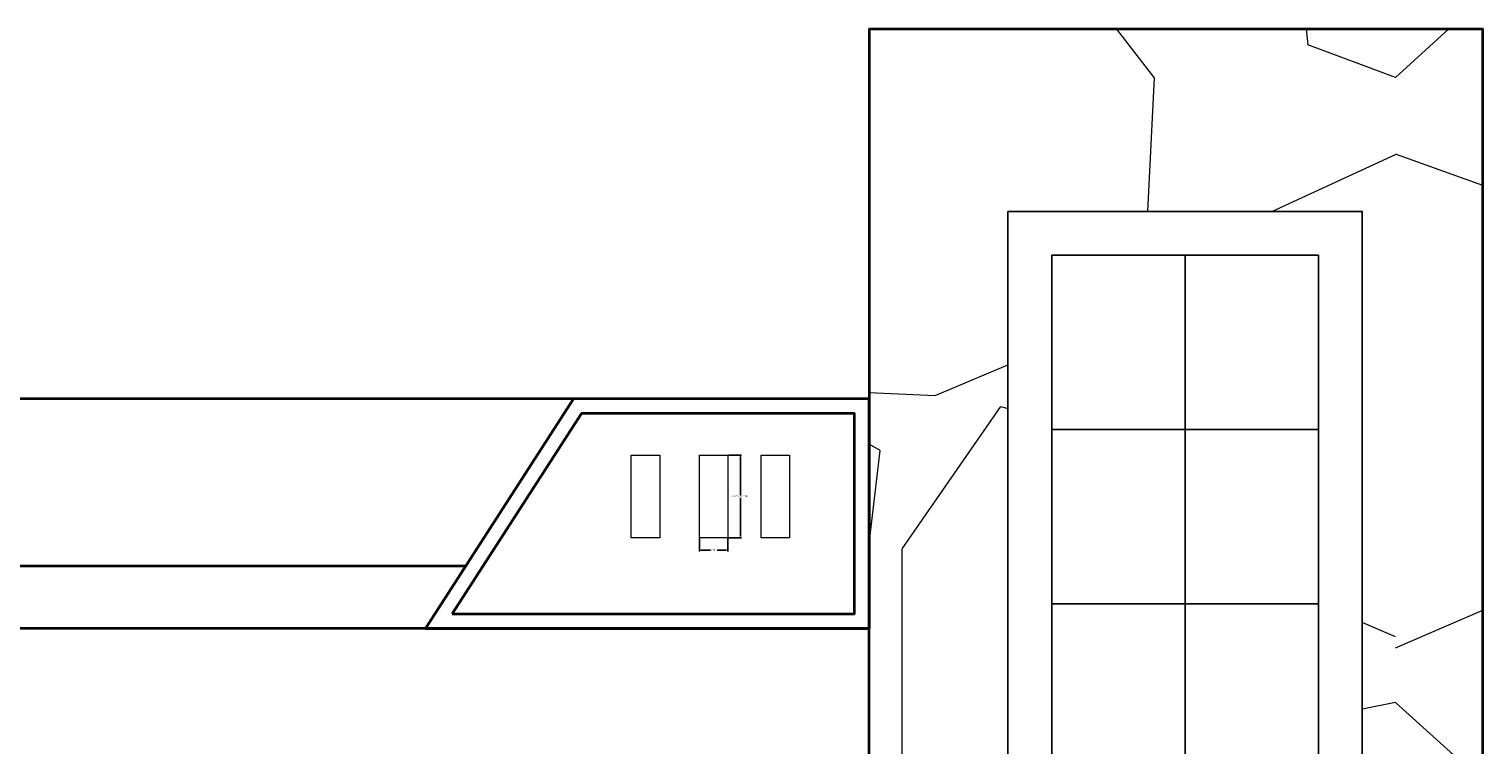
# Model space of a CAD drawing. Units: inches. Extents: x 3 to 303, y 4 to 326.
# Tile 6 of 6: x 104 to 303, y 228 to 326. Entities that reach past the tile are written whole.
import ezdxf

# ---------------------------------------------------------------- set-up
doc = ezdxf.new("R2010")
doc.units = ezdxf.units.IN
doc.header["$MEASUREMENT"] = 0
for name, color, linetype, lineweight in [('A-ANNO-DIMS', 2, 'Continuous', 18), ('A-ELEV', 7, 'Continuous', 35), ('A-ELEV-PATT', 8, 'Continuous', 13), ('A-ELEV-VENT', 4, 'Continuous', 18), ('A-GLAZ', 4, 'Continuous', 25)]:
    doc.layers.add(name, color=color, linetype=linetype, lineweight=lineweight)
doc.styles.get("Standard").update_dxf_attribs({"font": 'arial.ttf'})
doc.dimstyles.get("Standard").update_dxf_attribs({"dimtxt": 0.18, "dimasz": 0.18, "dimexe": 0.18, "dimexo": 0.0625, "dimgap": 0.09, "dimtad": 0, "dimtih": 1, "dimtoh": 1, "dimdec": 4, "dimzin": 0, "dimdsep": 46, "dimtxsty": 'Standard', "dimcen": 0.09, "dimadec": 0, "dimazin": 0, "dimtfac": 1, "dimtdec": 4, "dimtofl": 0, "dimtmove": 0, "dimatfit": 3, "dimfxl": 1, "dimtolj": 1, "dimtzin": 0, "dimarcsym": 0})

# ---------------------------------------------------------------- blocks, each defined once
blk = doc.blocks.new('VENT-SLOT')
blk.add_lwpolyline([(7.78475479422e-05, 11.31182104697234), (3.886723644854242, 11.31182104697234), (3.886723644854242, 0.0003310090934292), (7.78475479422e-05, 0.0003310090934292)], close=True)
blk = doc.blocks.new('*D8')
at = {"layer": 'A-ANNO-DIMS', "color": 0, "lineweight": -2, "transparency": 16777216}
for p, q in [((199.9722236448543, 267.3318210469724), (201.7864471505363, 267.3318210469724)), ((201.6064471505363, 267.1518210469724), (201.6064471505363, 261.8592069966551)), ((201.6064471505363, 256.2003310090935), (201.6064471505363, 261.4929450594109)), ((199.9722236448543, 256.0203310090935), (201.7864471505363, 256.0203310090935))]:
    blk.add_line(p, q, dxfattribs=at)
at = {"layer": 'A-ANNO-DIMS', "color": 0, "transparency": 16777216}
for points in [[(201.5764471505363, 267.1518210469724), (201.6364471505363, 267.1518210469724), (201.6064471505363, 267.3318210469724)], [(201.5764471505363, 256.2003310090935), (201.6364471505363, 256.2003310090935), (201.6064471505363, 256.0203310090935)]]:
    blk.add_solid(points, dxfattribs=at)
at = {"layer": 'Defpoints', "color": 0, "transparency": 16777216}
for p in [(199.9097236448543, 267.3318210469724), (201.6064471505363, 267.3318210469724), (199.9097236448543, 256.0203310090935)]:
    blk.add_point(p, dxfattribs=at)
at = {"layer": 'A-ANNO-DIMS', "color": 0, "transparency": 16777216, "insert": (201.6064471505363, 261.6760760280329), "char_height": 0.18, "attachment_point": 5}
blk.add_mtext('\\A1;VENT SLOT 11 TYP.', dxfattribs=at)
blk = doc.blocks.new('*D9')
at = {"layer": 'A-ANNO-DIMS', "color": 0, "lineweight": -2, "transparency": 16777216}
for p, q in [((196.0230778475479, 255.9578310090934), (196.0230778475479, 254.1436075034116)), ((199.9097236448542, 255.9578310090934), (199.9097236448542, 254.1436075034116)), ((196.2030778475479, 254.3236075034116), (197.504613570212, 254.3236075034116)), ((199.7297236448542, 254.3236075034116), (198.4281879221902, 254.3236075034116))]:
    blk.add_line(p, q, dxfattribs=at)
at = {"layer": 'A-ANNO-DIMS', "color": 0, "transparency": 16777216}
for points in [[(196.2030778475479, 254.3536075034116), (196.2030778475479, 254.2936075034116), (196.0230778475479, 254.3236075034116)], [(199.7297236448542, 254.3536075034116), (199.7297236448542, 254.2936075034116), (199.9097236448542, 254.3236075034116)]]:
    blk.add_solid(points, dxfattribs=at)
at = {"layer": 'Defpoints', "color": 0, "transparency": 16777216}
for p in [(196.0230778475479, 256.0203310090934), (199.9097236448542, 256.0203310090934), (199.9097236448542, 254.3236075034116)]:
    blk.add_point(p, dxfattribs=at)
at = {"layer": 'A-ANNO-DIMS', "color": 0, "transparency": 16777216, "insert": (197.9664007462011, 254.3236075034116), "char_height": 0.18, "attachment_point": 5}
blk.add_mtext('\\A1;4 TYP.', dxfattribs=at)

msp = doc.modelspace()

# ---------------------------------------------------------------- hatches: boundary and pattern name
at = {"layer": 'A-ELEV-PATT'}
h = msp.add_hatch(dxfattribs=at)
h.set_pattern_fill('GRAVEL', color=256, scale=150, angle=90)
h.set_pattern_definition([(318.012787504, (-159.711805372533, 82.49771926165387), (1350, -1200.000000000009), [20.1804, -1997.863207061055]), (274.969740728, (-144.711805372533, 68.99771926165387), (-150.0000000000051, 1799.999999999996), [34.6302, -3428.388714184499]), (222.510447078, (-141.711805372533, 34.49771926165386), (1649.99999999998, 1500.000000000017), [24.4182, -2417.404889414955]), (357.273689006, (-104.211805372533, -24.00228073834614), (-3000.000000000003, 150.0000000000038), [31.5357, -3122.03370624435]), (22.83365417800003, (-72.71180537253304, -25.50228073834614), (-1800.000000000004, -749.9999999999982), [30.92325, -3061.405969213245]), (87.27368900599996, (-44.21180537253303, -13.50228073834614), (-150.000000000004, -3000.000000000003), [31.5357, -3122.03370624435]), (127.6942404667, (-42.71180537253303, 17.99771926165385), (1499.999999999996, -1950), [41.70435, -4128.7272823374]), (162.2553283749, (-68.21180537253304, 50.99771926165385), (-3300.000000000001, 1050.000000000004), [39.3732, -3897.948224522009]), (211.429565615, (-105.711805372533, 62.99771926165385), (-1949.999999999998, -1200.000000000003), [31.6425, -3132.610966459349]), (265.236358309, (-132.711805372533, 46.49771926165387), (150.0000000000058, 1649.999999999997), [36.1248, -1770.114386818845]), (312.397437798, (-135.711805372533, 10.49771926165386), (1649.999999999996, -1799.999999999994), [46.71719999999999, -4625.006250719235]), (228.814074834, (-102.711805372533, 124.4977192616538), (-900.0000000000001, -1050.000000000005), [15.94515, -1578.576721910205]), (261.4692343899999, (-113.211805372533, 112.4977192616538), (299.9999999999994, 1950), [30.33555, -3003.22671242355]), (315, (-117.711805372533, 82.49771926165386), (149.9999999999899, -2.58e-14), [21.21315, -190.918884355965]), (293.198590514, (-135.711805372533, 71.99771926165387), (-299.9999999999963, 749.9999999999984), [11.4237, -1130.942265879585]), (21.80140948600004, (-131.211805372533, 61.49771926165387), (-450.0000000000154, -149.9999999999525), [16.15545, -791.619271070175]), (120.9637565321, (-116.211805372533, 67.49771926165386), (-299.9999999999969, 450.0000000000079), [26.23935, -848.4034342267948]), (251.565051177, (-129.711805372533, 89.99771926165387), (149.9999999999965, 300.0000000000017), [18.97365, -455.3679990252599]), (106.389540334, (-131.211805372533, -25.50228073834614), (-450.0000000000064, 1499.999999999995), [26.57999999999999, -2631.42677200041]), (160.3461759419, (-138.711805372533, -0.0022807383461334), (1650.000000000509, -600.0000000001831), [22.29915, -2207.61116209785]), (23.19859051399996, (-159.711805372533, 89.99771926165387), (-749.9999999999986, -299.9999999999955), [22.84725, -1119.518715879585]), (73.61045966600004, (-138.711805372533, 98.99771926165387), (-450.0000000000066, -1499.999999999995), [26.58, -2631.42677200035]), (69.44395478000004, (-38.21180537253304, -25.50228073834615), (-300.0000000000037, -750.0000000000055), [25.632, -1255.968561797625]), (24.775140569, (-29.21180537253304, -1.502280738346144), (-1650, -750.0000000000007), [21.4767, -2126.196459491399]), (156.8014094864, (-9.711805372533028, 91.49771926165386), (-749.9999999999955, 299.9999999999972), [22.84725, -1119.518715879585]), (107.3540246363, (-30.71180537253303, 100.4977192616538), (599.9999999999943, -1949.999999999997), [25.14465, -2489.313542136001]), (159.4439547804, (-9.711805372533034, 17.99771926165385), (749.9999999999931, -300.0000000000011), [12.816, -1268.784561797625]), (191.309932474, (-9.711805372533028, 82.49771926165386), (-600.0000000000018, -149.9999999999945), [7.6485, -757.2044270389199]), (255.963756532, (-17.21180537253303, 80.99771926165386), (150.0000000000002, 449.9999999999937), [30.92325, -587.542593842655]), (276.009005957, (-24.71180537253303, 50.99771926165385), (-149.9999999999974, 1500.000000000007), [28.6575, -2837.088476181421]), (33.69006752600001, (-102.711805372533, 67.49771926165386), (-299.9999999999979, -149.999999999998), [21.6333, -519.1993913196]), (83.15722658699998, (-84.71180537253304, 79.49771926165386), (300.0000000000081, 2550.000000000002), [37.7691, -3739.134393604246]), (150.9453959009, (-80.21180537253302, 116.9977192616538), (1049.999999999996, -599.9999999999964), [15.4434, -1528.90112114805]), (180, (-93.71180537253304, 124.4977192616538), (-150, -150), [9, -141]), (210.256437164, (-29.21180537253303, 47.99771926165385), (1050.000000000001, 600.0000000000013), [20.8386, -2063.02799841747]), (138.0127875042, (-47.21180537253302, 37.49771926165386), (-1349.999999999996, 1200), [40.3608, -1977.682807061055]), (90, (-77.21180537253304, 64.49771926165386), (-150, 150), [39, -111]), (55.30484646900005, (-77.21180537253302, 103.4977192616538), (1049.999999999974, 1500.000000000021), [23.7171, -2347.9911451263]), (344.054604099, (-63.71180537253303, 122.9977192616538), (600.0000000000007, -150.0000000000057), [21.8403, -1070.176183392075]), (297.645975364, (-42.71180537253303, 116.9977192616538), (1500.000000000007, -2849.999999999993), [35.55975, -3520.42112733891]), (265.42607874, (-26.21180537253303, 85.49771926165386), (-150.0000000000003, -1949.999999999993), [37.61985, -3724.361011195335])])
h.paths.add_polyline_path([(303.2262632093826, 123.6171748626421), (303.2262632093826, 243.6171748626422), (303.2262632093826, 325.612924607852), (219.2262632093826, 325.612924607852), (219.2262632093826, 243.6171748626422), (219.2262632093826, 63.61717486264215), (232.7289574534793, 63.61717486264215), (232.7289574534793, 80.06132969089668), (244.0693281795079, 80.06132969089668), (244.0693281795079, 63.61717486264215), (257.5720224236046, 63.61717486264215), (257.5720224236046, 80.06132969089668), (268.9123931496332, 80.06132969089668), (268.9123931496332, 63.61717486264215), (282.4150873937299, 63.61717486264214), (282.4150873937299, 80.06132969089668), (293.7554581197585, 80.06132969089668), (293.7554581197585, 63.61717486264215), (303.2262632093826, 63.61717486264215)])
h.paths.add_polyline_path([(286.7238180358027, 105.3811659699868), (238.2183155441071, 105.3811659699868), (238.2183155441071, 300.6586406846385), (286.7238180358027, 300.6586406846385)], flags=16)
h.paths.add_polyline_path([(280.7238180358027, 111.3811659699868), (244.2183155441071, 111.3811659699868), (244.2183155441071, 294.6586406846385), (280.7238180358027, 294.6586406846385)], flags=0)

# ---------------------------------------------------------------- linework, layer by layer
at = {"layer": 'A-ELEV'}
for p, q in [((178.7916742773327, 275.0276219683291), (87.22626320938262, 275.0276219683291)), ((164.0138881640637, 252.1264006774053), (15.22626320938263, 252.1264006774053)), ((219.2262632093826, 243.6171748626422), (15.22626320938262, 243.6171748626422)), ((219.2262632093826, 3.617174862642144), (219.2262632093826, 243.6171748626422)), ((303.2262632093826, 123.6171748626421), (303.2262632093826, 243.6171748626422))]:
    msp.add_line(p, q, dxfattribs=at)
msp.add_lwpolyline([(303.2262632093826, 243.6171748626422), (303.2262632093826, 325.612924607852), (219.2262632093826, 325.612924607852), (219.2262632093826, 243.6171748626422)], dxfattribs=at)
for points in [[(158.5230229616077, 243.6171748626421), (219.2262632093826, 243.6171748626421), (219.2262632093826, 275.0276219683291), (178.7916742773327, 275.0276219683291)], [(162.1938351074482, 245.6171748626421), (217.2262632093826, 245.6171748626421), (217.2262632093826, 273.0276219683291), (179.8813513953875, 273.0276219683291)]]:
    msp.add_lwpolyline(points, close=True, dxfattribs=at)
at = {"layer": 'A-GLAZ'}
for p, q in [((262.4710667899549, 294.6586406846385), (262.4710667899549, 111.3811659699868)), ((244.2183155441071, 270.8084808110744), (280.7238180358027, 270.8084808110744)), ((244.2183155441071, 246.9583209375104), (280.7238180358027, 246.9583209375104))]:
    msp.add_line(p, q, dxfattribs=at)
for points in [[(238.2183155441071, 300.6586406846385), (286.7238180358027, 300.6586406846385), (286.7238180358027, 105.3811659699868), (238.2183155441071, 105.3811659699868)], [(244.2183155441071, 294.6586406846385), (280.7238180358027, 294.6586406846385), (280.7238180358027, 111.3811659699868), (244.2183155441071, 111.3811659699868)]]:
    msp.add_lwpolyline(points, close=True, dxfattribs=at)

# ---------------------------------------------------------------- block references
at = {"layer": 'A-ELEV-VENT'}
for p in [(186.6807238224682, 256.02), (196.023, 256.02), (204.4397598759587, 256.02)]:
    msp.add_blockref('VENT-SLOT', p, dxfattribs=at)

# ---------------------------------------------------------------- dimensions: what is measured, and where the dimension line sits
at = {"layer": 'A-ANNO-DIMS'}
dim = msp.add_linear_dim(base=(201.6064471505363, 267.3318210469724), p1=(199.9097236448542, 256.0203310090934), p2=(199.9097236448542, 267.3318210469723), angle=90, text='VENT SLOT <> TYP.', dimstyle='Standard', override={"dimdec": 0, "dimlfac": 1, "dimrnd": 0, "dimzin": 0, "dimdsep": 46, "dimlunit": 2}, dxfattribs=at)
dim.commit()
dim.dimension.update_dxf_attribs({"geometry": '*D8', "text_midpoint": (201.6064471505363, 261.6760760280329)})
dim = msp.add_linear_dim(base=(199.9097236448542, 254.3236075034116), p1=(196.0230778475479, 256.0203310090934), p2=(199.9097236448542, 256.0203310090934), text='<> TYP.', dimstyle='Standard', override={"dimdec": 0, "dimlfac": 1, "dimrnd": 0, "dimzin": 0, "dimdsep": 46, "dimlunit": 2}, dxfattribs=at)
dim.commit()
dim.dimension.update_dxf_attribs({"geometry": '*D9', "text_midpoint": (197.9664007462011, 254.3236075034116)})

doc.saveas('drawing.dxf')
